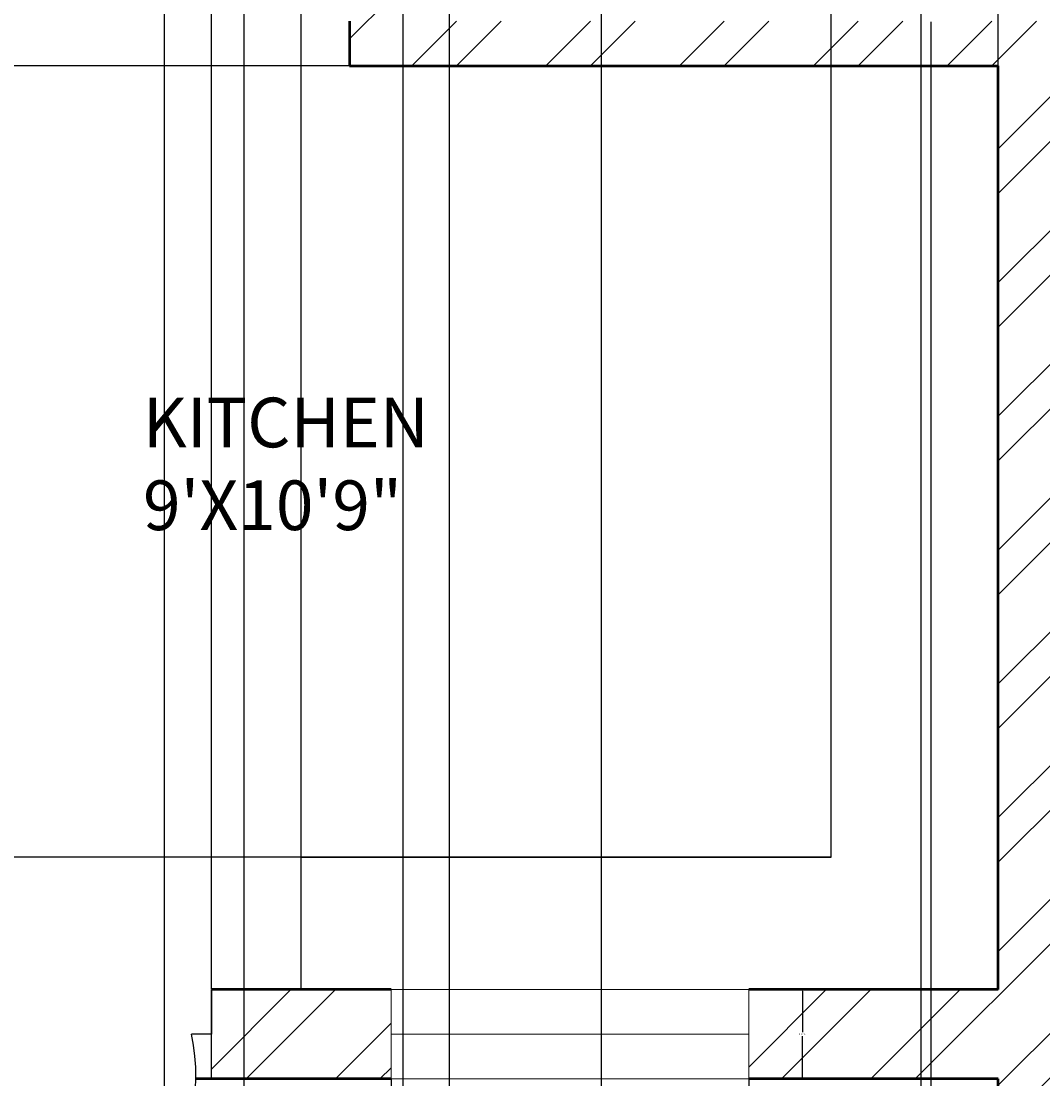
# Model space of a CAD drawing. Units: inches. Extents: x 1980 to 2738, y 1471 to 2568.
# Tile 5 of 22: x 2260 to 2363, y 1686 to 1792. Entities that reach past the tile are written whole.
import ezdxf

# ---------------------------------------------------------------- set-up
doc = ezdxf.new("R2010")
doc.units = ezdxf.units.IN
for name, color, linetype, lineweight in [('A-ANNO-DIMS', 2, 'Continuous', 18), ('A-AREA-IDEN', 7, 'Continuous', 18), ('A-DOOR', 31, 'Continuous', 25), ('A-FLOR-CASE', 8, 'Continuous', 25), ('A-GLAZ', 141, 'Continuous', 18), ('A-WALL', 7, 'Continuous', 50)]:
    doc.layers.add(name, color=color, linetype=linetype, lineweight=lineweight)
doc.layers.add('A-WALL-PATT', color=9, linetype='Continuous', lineweight=13, true_color=0xd19cc7)
doc.styles.get("Standard").update_dxf_attribs({"font": 'arial.ttf'})
doc.dimstyles.get("Standard").update_dxf_attribs({"dimtxt": 0.18, "dimasz": 0.18, "dimexe": 0.18, "dimexo": 0.0625, "dimgap": 0.09, "dimtad": 0, "dimtih": 1, "dimtoh": 1, "dimdec": 4, "dimzin": 0, "dimdsep": 46, "dimtxsty": 'Standard', "dimcen": 0.09, "dimadec": 0, "dimazin": 0, "dimtfac": 1, "dimtdec": 4, "dimtofl": 0, "dimtmove": 0, "dimatfit": 3, "dimfxl": 1, "dimtolj": 1, "dimtzin": 0, "dimarcsym": 0})

# ---------------------------------------------------------------- blocks, each defined once
blk = doc.blocks.new('WIN-36IN-WALL')
for p, q in [((0, 9), (0, 0)), ((0, 9), (36, 9)), ((36, 4.5), (36, 9)), ((36, 9), (36, 0)), ((0, 0), (0, 4.5)), ((0, 4.5), (36, 4.5)), ((36, 0), (0, 0))]:
    blk.add_line(p, q)
blk = doc.blocks.new('*D31')
at = {"layer": 'A-ANNO-DIMS', "color": 0, "lineweight": -2, "transparency": 16777216}
for p, q in [((2297.48, 1685.64), (2297.48, 1680.13)), ((2333.48, 1685.64), (2333.48, 1680.13)), ((2297.66, 1680.31), (2314.36, 1680.31)), ((2333.3, 1680.31), (2316.59, 1680.31))]:
    blk.add_line(p, q, dxfattribs=at)
at = {"layer": 'A-ANNO-DIMS', "color": 0, "transparency": 16777216}
for points in [[(2297.66, 1680.34), (2297.66, 1680.28), (2297.48, 1680.31)], [(2333.3, 1680.34), (2333.3, 1680.28), (2333.48, 1680.31)]]:
    blk.add_solid(points, dxfattribs=at)
at = {"layer": 'Defpoints', "color": 0, "transparency": 16777216}
for p in [(2297.48, 1685.71), (2333.48, 1685.71), (2333.48, 1680.31)]:
    blk.add_point(p, dxfattribs=at)
at = {"layer": 'A-ANNO-DIMS', "color": 0, "transparency": 16777216, "insert": (2315.48, 1680.31), "char_height": 0.18, "attachment_point": 5}
blk.add_mtext('\\A1;WINDOW 36 TYP.', dxfattribs=at)
blk = doc.blocks.new('*D32')
at = {"layer": 'A-ANNO-DIMS', "color": 0, "lineweight": -2, "transparency": 16777216}
for p, q in [((2333.54, 1694.71), (2339.06, 1694.71)), ((2338.88, 1694.53), (2338.88, 1690.39)), ((2338.88, 1685.89), (2338.88, 1690.02)), ((2333.54, 1685.71), (2339.06, 1685.71))]:
    blk.add_line(p, q, dxfattribs=at)
at = {"layer": 'A-ANNO-DIMS', "color": 0, "transparency": 16777216}
for points in [[(2338.85, 1694.53), (2338.91, 1694.53), (2338.88, 1694.71)], [(2338.85, 1685.89), (2338.91, 1685.89), (2338.88, 1685.71)]]:
    blk.add_solid(points, dxfattribs=at)
at = {"layer": 'Defpoints', "color": 0, "transparency": 16777216}
for p in [(2333.48, 1694.71), (2338.88, 1694.71), (2333.48, 1685.71)]:
    blk.add_point(p, dxfattribs=at)
at = {"layer": 'A-ANNO-DIMS', "color": 0, "transparency": 16777216, "insert": (2338.88, 1690.21), "char_height": 0.18, "attachment_point": 5}
blk.add_mtext('\\A1;9 TYP.', dxfattribs=at)
blk = doc.blocks.new('*D40')
at = {"layer": 'A-ANNO-DIMS', "color": 0, "lineweight": -2, "transparency": 16777216}
for p, q in [((2218.65, 2053.14), (2218.65, 1533.71)), ((2298.65, 2053.14), (2298.65, 1533.71)), ((2218.83, 1533.89), (2258.43, 1533.89)), ((2298.47, 1533.89), (2258.87, 1533.89))]:
    blk.add_line(p, q, dxfattribs=at)
at = {"layer": 'A-ANNO-DIMS', "color": 0, "transparency": 16777216}
for points in [[(2218.83, 1533.92), (2218.83, 1533.86), (2218.65, 1533.89)], [(2298.47, 1533.92), (2298.47, 1533.86), (2298.65, 1533.89)]]:
    blk.add_solid(points, dxfattribs=at)
at = {"layer": 'Defpoints', "color": 0, "transparency": 16777216}
for p in [(2218.65, 2053.21), (2298.65, 2053.21), (2298.65, 1533.89)]:
    blk.add_point(p, dxfattribs=at)
at = {"layer": 'A-ANNO-DIMS', "color": 0, "transparency": 16777216, "insert": (2258.65, 1533.89), "char_height": 0.18, "attachment_point": 5}
blk.add_mtext('\\A1;80', dxfattribs=at)
blk = doc.blocks.new('*D41')
at = {"layer": 'A-ANNO-DIMS', "color": 0, "lineweight": -2, "transparency": 16777216}
for p, q in [((2298.65, 2095.14), (2298.65, 1533.71)), ((2515.4, 2095.14), (2515.4, 1533.71)), ((2298.83, 1533.89), (2406.56, 1533.89)), ((2515.22, 1533.89), (2407.49, 1533.89))]:
    blk.add_line(p, q, dxfattribs=at)
at = {"layer": 'A-ANNO-DIMS', "color": 0, "transparency": 16777216}
for points in [[(2298.83, 1533.92), (2298.83, 1533.86), (2298.65, 1533.89)], [(2515.22, 1533.92), (2515.22, 1533.86), (2515.4, 1533.89)]]:
    blk.add_solid(points, dxfattribs=at)
at = {"layer": 'Defpoints', "color": 0, "transparency": 16777216}
for p in [(2298.65, 2095.21), (2515.4, 2095.21), (2515.4, 1533.89)]:
    blk.add_point(p, dxfattribs=at)
at = {"layer": 'A-ANNO-DIMS', "color": 0, "transparency": 16777216, "insert": (2407.03, 1533.89), "char_height": 0.18, "attachment_point": 5}
blk.add_mtext('\\A1;216.75', dxfattribs=at)
blk = doc.blocks.new('*D45')
at = {"layer": 'A-ANNO-DIMS', "color": 0, "lineweight": -2, "transparency": 16777216}
for p, q in [((2255.99, 1694.77), (2255.99, 2507.54)), ((2256.17, 2507.36), (2267.22, 2507.36)), ((2279.21, 2507.36), (2268.15, 2507.36)), ((2279.39, 1694.77), (2279.39, 2507.54))]:
    blk.add_line(p, q, dxfattribs=at)
at = {"layer": 'A-ANNO-DIMS', "color": 0, "transparency": 16777216}
for points in [[(2256.17, 2507.39), (2256.17, 2507.33), (2255.99, 2507.36)], [(2279.21, 2507.39), (2279.21, 2507.33), (2279.39, 2507.36)]]:
    blk.add_solid(points, dxfattribs=at)
at = {"layer": 'Defpoints', "color": 0, "transparency": 16777216}
for p in [(2279.39, 2507.36), (2255.99, 1694.71), (2279.39, 1694.71)]:
    blk.add_point(p, dxfattribs=at)
at = {"layer": 'A-ANNO-DIMS', "color": 0, "transparency": 16777216, "insert": (2267.69, 2507.36), "char_height": 0.18, "attachment_point": 5}
blk.add_mtext('\\A1;23.407', dxfattribs=at)
blk = doc.blocks.new('*D50')
at = {"layer": 'A-ANNO-DIMS', "color": 0, "lineweight": -2, "transparency": 16777216}
for p, q in [((2288.43, 1708.09), (2288.43, 2507.54)), ((2288.61, 2507.36), (2314.71, 2507.36)), ((2341.6, 2507.36), (2315.5, 2507.36)), ((2341.78, 1708.09), (2341.78, 2507.54))]:
    blk.add_line(p, q, dxfattribs=at)
at = {"layer": 'A-ANNO-DIMS', "color": 0, "transparency": 16777216}
for points in [[(2288.61, 2507.39), (2288.61, 2507.33), (2288.43, 2507.36)], [(2341.6, 2507.39), (2341.6, 2507.33), (2341.78, 2507.36)]]:
    blk.add_solid(points, dxfattribs=at)
at = {"layer": 'Defpoints', "color": 0, "transparency": 16777216}
for p in [(2341.78, 2507.36), (2288.43, 1708.03), (2341.78, 1708.03)]:
    blk.add_point(p, dxfattribs=at)
at = {"layer": 'A-ANNO-DIMS', "color": 0, "transparency": 16777216, "insert": (2315.11, 2507.36), "char_height": 0.18, "attachment_point": 5}
blk.add_mtext('\\A1;53.34', dxfattribs=at)
blk = doc.blocks.new('*D51')
at = {"layer": 'A-ANNO-DIMS', "color": 0, "lineweight": -2, "transparency": 16777216}
for p, q in [((2341.78, 1708.09), (2341.78, 2507.54)), ((2341.96, 2507.36), (2349.72, 2507.36)), ((2358.4, 2507.36), (2350.63, 2507.36)), ((2358.58, 1694.77), (2358.58, 2507.54))]:
    blk.add_line(p, q, dxfattribs=at)
at = {"layer": 'A-ANNO-DIMS', "color": 0, "transparency": 16777216}
for points in [[(2341.96, 2507.39), (2341.96, 2507.33), (2341.78, 2507.36)], [(2358.4, 2507.39), (2358.4, 2507.33), (2358.58, 2507.36)]]:
    blk.add_solid(points, dxfattribs=at)
at = {"layer": 'Defpoints', "color": 0, "transparency": 16777216}
for p in [(2358.58, 2507.36), (2341.78, 1708.03), (2358.58, 1694.71)]:
    blk.add_point(p, dxfattribs=at)
at = {"layer": 'A-ANNO-DIMS', "color": 0, "transparency": 16777216, "insert": (2350.18, 2507.36), "char_height": 0.18, "attachment_point": 5}
blk.add_mtext('\\A1;16.807', dxfattribs=at)
blk = doc.blocks.new('*D52')
at = {"layer": 'A-ANNO-DIMS', "color": 0, "lineweight": -2, "transparency": 16777216}
for p, q in [((2341.71, 1787.71), (2036.25, 1787.71)), ((2036.43, 1787.53), (2036.43, 1748.05)), ((2036.43, 1708.21), (2036.43, 1747.69)), ((2341.71, 1708.03), (2036.25, 1708.03))]:
    blk.add_line(p, q, dxfattribs=at)
at = {"layer": 'A-ANNO-DIMS', "color": 0, "transparency": 16777216}
for points in [[(2036.4, 1787.53), (2036.46, 1787.53), (2036.43, 1787.71)], [(2036.4, 1708.21), (2036.46, 1708.21), (2036.43, 1708.03)]]:
    blk.add_solid(points, dxfattribs=at)
at = {"layer": 'Defpoints', "color": 0, "transparency": 16777216}
for p in [(2036.43, 1787.71), (2341.78, 1787.71), (2341.78, 1708.03)]:
    blk.add_point(p, dxfattribs=at)
at = {"layer": 'A-ANNO-DIMS', "color": 0, "transparency": 16777216, "insert": (2036.43, 1747.87), "char_height": 0.18, "attachment_point": 5}
blk.add_mtext('\\A1;79.68', dxfattribs=at)
blk = doc.blocks.new('*D53')
at = {"layer": 'A-ANNO-DIMS', "color": 0, "lineweight": -2, "transparency": 16777216}
for p, q in [((2318.63, 2002.14), (2318.63, 1533.71)), ((2350.79, 2002.14), (2350.79, 1533.71)), ((2318.81, 1533.89), (2334.25, 1533.89)), ((2350.61, 1533.89), (2335.18, 1533.89))]:
    blk.add_line(p, q, dxfattribs=at)
at = {"layer": 'A-ANNO-DIMS', "color": 0, "transparency": 16777216}
for points in [[(2318.81, 1533.92), (2318.81, 1533.86), (2318.63, 1533.89)], [(2350.61, 1533.92), (2350.61, 1533.86), (2350.79, 1533.89)]]:
    blk.add_solid(points, dxfattribs=at)
at = {"layer": 'Defpoints', "color": 0, "transparency": 16777216}
for p in [(2318.63, 2002.21), (2350.79, 2002.21), (2350.79, 1533.89)]:
    blk.add_point(p, dxfattribs=at)
at = {"layer": 'A-ANNO-DIMS', "color": 0, "transparency": 16777216, "insert": (2334.71, 1533.89), "char_height": 0.18, "attachment_point": 5}
blk.add_mtext('\\A1;32.155', dxfattribs=at)
blk = doc.blocks.new('*D57')
at = {"layer": 'A-ANNO-DIMS', "color": 0, "lineweight": -2, "transparency": 16777216}
for p, q in [((2351.81, 1792.14), (2351.81, 1533.71)), ((2372.53, 1792.14), (2372.53, 1533.71)), ((2351.99, 1533.89), (2361.77, 1533.89)), ((2372.35, 1533.89), (2362.56, 1533.89))]:
    blk.add_line(p, q, dxfattribs=at)
at = {"layer": 'A-ANNO-DIMS', "color": 0, "transparency": 16777216}
for points in [[(2351.99, 1533.92), (2351.99, 1533.86), (2351.81, 1533.89)], [(2372.35, 1533.92), (2372.35, 1533.86), (2372.53, 1533.89)]]:
    blk.add_solid(points, dxfattribs=at)
at = {"layer": 'Defpoints', "color": 0, "transparency": 16777216}
for p in [(2351.81, 1792.21), (2372.53, 1792.21), (2372.53, 1533.89)]:
    blk.add_point(p, dxfattribs=at)
at = {"layer": 'A-ANNO-DIMS', "color": 0, "transparency": 16777216, "insert": (2362.17, 1533.89), "char_height": 0.18, "attachment_point": 5}
blk.add_mtext('\\A1;20.72', dxfattribs=at)
blk = doc.blocks.new('*D64')
at = {"layer": 'A-ANNO-DIMS', "color": 0, "lineweight": -2, "transparency": 16777216}
for p, q in [((2303.33, 2002.14), (2303.33, 1533.71)), ((2318.63, 2002.14), (2318.63, 1533.71)), ((2303.51, 1533.89), (2310.67, 1533.89)), ((2318.45, 1533.89), (2311.3, 1533.89))]:
    blk.add_line(p, q, dxfattribs=at)
at = {"layer": 'A-ANNO-DIMS', "color": 0, "transparency": 16777216}
for points in [[(2303.51, 1533.92), (2303.51, 1533.86), (2303.33, 1533.89)], [(2318.45, 1533.92), (2318.45, 1533.86), (2318.63, 1533.89)]]:
    blk.add_solid(points, dxfattribs=at)
at = {"layer": 'Defpoints', "color": 0, "transparency": 16777216}
for p in [(2303.33, 2002.21), (2318.63, 2002.21), (2318.63, 1533.89)]:
    blk.add_point(p, dxfattribs=at)
at = {"layer": 'A-ANNO-DIMS', "color": 0, "transparency": 16777216, "insert": (2310.98, 1533.89), "char_height": 0.18, "attachment_point": 5}
blk.add_mtext('\\A1;15.3', dxfattribs=at)
blk = doc.blocks.new('*D66')
at = {"layer": 'A-ANNO-DIMS', "color": 0, "lineweight": -2, "transparency": 16777216}
for p, q in [((2274.65, 2095.14), (2274.65, 1533.71)), ((2282.65, 2095.14), (2282.65, 1533.71)), ((2274.83, 1533.89), (2278.5, 1533.89)), ((2282.47, 1533.89), (2278.8, 1533.89))]:
    blk.add_line(p, q, dxfattribs=at)
at = {"layer": 'A-ANNO-DIMS', "color": 0, "transparency": 16777216}
for points in [[(2274.83, 1533.92), (2274.83, 1533.86), (2274.65, 1533.89)], [(2282.47, 1533.92), (2282.47, 1533.86), (2282.65, 1533.89)]]:
    blk.add_solid(points, dxfattribs=at)
at = {"layer": 'Defpoints', "color": 0, "transparency": 16777216}
for p in [(2274.65, 2095.21), (2282.65, 2095.21), (2282.65, 1533.89)]:
    blk.add_point(p, dxfattribs=at)
at = {"layer": 'A-ANNO-DIMS', "color": 0, "transparency": 16777216, "insert": (2278.65, 1533.89), "char_height": 0.18, "attachment_point": 5}
blk.add_mtext('\\A1;8', dxfattribs=at)

msp = doc.modelspace()

# ---------------------------------------------------------------- hatches: boundary and pattern name
at = {"layer": 'A-WALL-PATT'}
h = msp.add_hatch(dxfattribs=at)
h.set_pattern_fill('ANSI32', color=256)
h.paths.add_polyline_path([(2257.5661, 2416.2064), (2257.5661, 2420.7064), (2250.5833, 2420.7064), (2250.5833, 2462.7064), (2246.0833, 2462.7064), (2246.0833, 2420.7064), (2237.0791, 2420.7064), (2237.0791, 2411.7064), (2246.0833, 2411.7064), (2246.0833, 2291.7064), (2242.6109, 2291.7064), (2242.6109, 2287.2064), (2246.0833, 2287.2064), (2250.5833, 2287.2064), (2250.5833, 2291.7064), (2250.5833, 2411.7064), (2257.5661, 2411.7064)])
h.paths.add_polyline_path([(2387.0396, 2416.2064), (2387.0396, 2420.7064), (2367.5833, 2420.7064), (2367.5833, 2462.7064), (2358.5833, 2462.7064), (2358.5833, 2420.7064), (2329.3087, 2420.7064), (2329.3087, 2411.7064), (2358.5833, 2411.7064), (2358.5833, 2321.7275), (2358.5833, 2309.7064), (2347.3089, 2309.7064), (2293.3089, 2309.7064), (2293.3089, 2259.0771), (2297.8089, 2259.0771), (2297.8089, 2305.2064), (2347.3089, 2305.2064), (2347.3089, 2284.7412), (2351.8089, 2284.7412), (2351.8089, 2305.2064), (2372.3188, 2305.2064), (2372.3761, 2284.3899), (2377.0295, 2284.3899), (2377.0295, 2299.3058), (2377.0295, 2305.2064), (2426.5295, 2305.2064), (2426.5295, 2257.5573), (2431.0295, 2257.5573), (2431.0295, 2309.7064), (2377.0295, 2309.7064), (2367.5833, 2309.7064), (2367.5833, 2321.7275), (2367.5833, 2411.7064), (2387.0396, 2411.7064)])
h.paths.add_polyline_path([(2448.5267, 2416.2064), (2448.5267, 2420.7064), (2423.0396, 2420.7064), (2423.0396, 2411.7064), (2448.5267, 2411.7064)])
h.paths.add_polyline_path([(2130.9128, 2416.2064), (2130.9128, 2420.7064), (2105.0833, 2420.7064), (2105.0833, 2386.6942), (2114.0833, 2386.6942), (2114.0833, 2411.7064), (2130.9128, 2411.7064)])
h.paths.add_polyline_path([(2212.9478, 2420.7064), (2190.9128, 2420.7064), (2190.9128, 2411.7064), (2212.9478, 2411.7064), (2212.9478, 2416.2064)])
h.paths.add_polyline_path([(2114.0833, 2326.6942), (2105.0833, 2326.6942), (2105.0833, 2291.7064), (2081.0833, 2291.7064), (2081.0833, 2287.2064), (2105.0833, 2287.2064), (2105.0833, 2276.1935), (2114.0833, 2276.1935), (2114.0833, 2287.2064), (2166.3825, 2287.2064), (2166.3825, 2289.4564), (2166.3825, 2291.7064), (2114.0833, 2291.7064)])
h.paths.add_polyline_path([(2114.0833, 2252.1935), (2105.0833, 2252.1935), (2105.0833, 2233.2064), (2081.0833, 2233.2064), (2081.0833, 2228.7064), (2105.0833, 2228.7064), (2105.0833, 2213.4478), (2114.0833, 2213.4478), (2114.0833, 2228.7064), (2195.0833, 2228.7064), (2199.5833, 2228.7064), (2208.4455, 2228.7064), (2208.4455, 2230.9564), (2208.4455, 2233.2064), (2199.5833, 2233.2064), (2199.5833, 2287.2064), (2206.8904, 2287.2064), (2206.8904, 2289.4564), (2206.8904, 2291.7064), (2189.446, 2291.7064), (2189.446, 2289.4564), (2189.446, 2287.2064), (2195.0833, 2287.2064), (2195.0833, 2233.2064), (2114.0833, 2233.2064)])
h.paths.add_polyline_path([(2114.0833, 2153.4478), (2109.5833, 2153.4478), (2105.0833, 2153.4478), (2105.0833, 2135.2374), (2114.0833, 2135.2374)], flags=17)
h.paths.add_polyline_path([(2135.9619, 2095.4081), (2140.1805, 2095.4081), (2140.1805, 2104.2064), (2114.0833, 2104.2064), (2114.0833, 2110.3997), (2109.5833, 2110.3997), (2105.0833, 2110.3997), (2105.0833, 2104.2064), (2081.0833, 2104.2064), (2081.0833, 2099.7064), (2105.0833, 2099.7064), (2127.5416, 2099.8532), (2127.5416, 2056.9393), (2136.2133, 2056.9393)], flags=17)
h.paths.add_polyline_path([(2255.4895, 2104.2064), (2250.5833, 2104.2064), (2250.5833, 2233.2064), (2246.0833, 2233.2064), (2242.4941, 2233.2064), (2242.4941, 2228.7064), (2246.0833, 2228.7064), (2246.0833, 2104.2064), (2163.6825, 2104.2064), (2163.6825, 2099.8072), (2163.6825, 2095.4081), (2191.4325, 2095.4081), (2191.4325, 2011.2064), (2186.0833, 2011.2064), (2136.5143, 2010.8824), (2136.3702, 2032.9403), (2131.9559, 2032.9115), (2127.5416, 2032.8826), (2127.5416, 2006.7064), (2105.0833, 2006.7064), (2081.0833, 2006.7064), (2081.0833, 2002.2064), (2105.0833, 2002.2064), (2105.0833, 1995.9329), (2114.0833, 1995.9329), (2114.0833, 2002.2064), (2246.0833, 2002.2064), (2246.0833, 1877.7064), (2242.1358, 1877.7064), (2242.1358, 1873.2064), (2250.5833, 1873.2064), (2250.5833, 2002.2064), (2255.3335, 2002.2064), (2255.3335, 2011.2064), (2195.9325, 2011.2064), (2195.9325, 2095.2064), (2255.4895, 2095.2064), (2255.4895, 2099.5471)])
h.paths.add_polyline_path([(2199.5833, 1873.2064), (2209.827, 1873.2064), (2209.827, 1875.4564), (2209.827, 1877.7064), (2114.0833, 1877.7064), (2114.0833, 1890.0968), (2105.0833, 1890.0968), (2105.0833, 1877.7064), (2081.0833, 1877.7064), (2081.0833, 1873.2064), (2105.0833, 1873.2064), (2105.0833, 1857.7279), (2114.0833, 1857.7279), (2114.0833, 1873.2064), (2195.0833, 1873.2064), (2195.0833, 1819.2064), (2190.298, 1819.2064), (2190.298, 1814.7064), (2209.8976, 1814.7064), (2209.8976, 1816.9564), (2209.8976, 1819.2064), (2199.5833, 1819.2064)])
h.paths.add_polyline_path([(2114.0833, 1814.7064), (2166.2538, 1814.7064), (2166.2538, 1816.9564), (2166.2538, 1819.2064), (2114.0833, 1819.2064), (2114.0833, 1833.7279), (2109.5833, 1833.7279), (2105.0833, 1833.7279), (2105.0833, 1819.2064), (2081.0833, 1819.2064), (2081.0833, 1814.7064), (2105.0833, 1814.7064), (2105.0833, 1782.5516), (2114.0833, 1782.5516)])
h.paths.add_polyline_path([(2114.0833, 1722.5516), (2109.5833, 1722.5516), (2105.0833, 1722.5516), (2105.0833, 1685.7064), (2124.5104, 1685.7064), (2124.5104, 1690.2064), (2124.5104, 1694.7064), (2114.0833, 1694.7064)])
h.paths.add_polyline_path([(2218.8787, 1694.7064), (2184.5104, 1694.7064), (2184.5104, 1685.7064), (2218.8787, 1685.7064), (2218.8787, 1690.2064)])
h.paths.add_polyline_path([(2250.5833, 1819.2064), (2242.6431, 1819.2064), (2242.6431, 1816.9564), (2242.6431, 1814.7064), (2246.0833, 1814.7064), (2246.0833, 1694.7064), (2240.4035, 1694.7064), (2240.4035, 1690.2064), (2240.4035, 1685.7064), (2246.0833, 1685.7064), (2246.0833, 1643.7064), (2250.5833, 1643.7064), (2250.5833, 1685.7064), (2255.9859, 1685.7064), (2255.9859, 1690.2064), (2255.9859, 1694.7064), (2250.5833, 1694.7064)])
h.paths.add_polyline_path([(2297.4764, 1694.7064), (2279.3934, 1694.7064), (2279.3934, 1690.2064), (2279.3934, 1685.7064), (2297.4764, 1685.7064), (2297.4764, 1690.2064)])
h.paths.add_polyline_path([(2377.1596, 1694.7064), (2367.5833, 1694.7064), (2367.5833, 1787.7064), (2431.0295, 1787.7064), (2431.0295, 1792.2064), (2431.0295, 1849.4149), (2428.7795, 1849.4149), (2426.5295, 1849.4149), (2426.5295, 1792.2064), (2421.5833, 1792.2064), (2367.5833, 1792.2064), (2297.8089, 1792.2064), (2297.8089, 1850.2946), (2295.5589, 1850.2946), (2293.3089, 1850.2946), (2293.3089, 1792.2064), (2293.3089, 1787.7064), (2297.8089, 1787.7064), (2358.5833, 1787.7064), (2358.5833, 1694.7064), (2333.4764, 1694.7064), (2333.4764, 1685.7064), (2358.5833, 1685.7064), (2358.5833, 1643.7064), (2367.5833, 1643.7064), (2367.5833, 1685.7064), (2377.1596, 1685.7064)])
h.paths.add_polyline_path([(2442.4912, 1694.7064), (2413.1596, 1694.7064), (2413.1596, 1685.7064), (2442.4912, 1685.7064)])
h.paths.add_polyline_path([(2480.0833, 1814.7064), (2483.4816, 1814.7064), (2483.4816, 1817.9384), (2483.4816, 1819.2064), (2475.5833, 1819.2064), (2475.5833, 1694.7064), (2470.7283, 1694.7064), (2470.7283, 1685.7064), (2475.5833, 1685.7064), (2475.5833, 1643.7064), (2480.0833, 1643.7064), (2480.0833, 1685.7064), (2486.3293, 1685.7064), (2486.3293, 1690.2064), (2486.3293, 1694.7064), (2480.0833, 1694.7064)])
h.paths.add_polyline_path([(2621.0833, 1721.7349), (2612.0833, 1721.7349), (2612.0833, 1694.7064), (2586.1453, 1694.7064), (2586.1453, 1685.7064), (2621.0833, 1685.7064)])
h.paths.add_polyline_path([(2526.1453, 1690.2064), (2526.1453, 1694.7064), (2511.584, 1694.7064), (2511.584, 1690.2064), (2511.584, 1685.7064), (2526.1453, 1685.7064)])
h.paths.add_polyline_path([(2645.0833, 1819.2064), (2621.0833, 1819.2064), (2621.0833, 1835.8527), (2616.5833, 1835.8527), (2612.0833, 1835.8527), (2612.0833, 1819.2064), (2560.2541, 1819.2064), (2560.2541, 1814.7064), (2612.0833, 1814.7064), (2612.0833, 1781.7349), (2621.0833, 1781.7349), (2621.0833, 1814.7064), (2645.0833, 1814.7064)])
h.paths.add_polyline_path([(2645.0833, 1877.7064), (2621.0833, 1877.7064), (2621.0833, 1886.4375), (2612.0833, 1886.4375), (2612.0833, 1877.7064), (2517.1032, 1877.7064), (2517.1032, 1875.4564), (2517.1032, 1873.2064), (2526.5833, 1873.2064), (2526.5833, 1819.2064), (2516.6454, 1819.2064), (2516.6454, 1816.9564), (2516.6454, 1814.7064), (2536.4445, 1814.7064), (2536.4445, 1816.9564), (2536.4445, 1819.2064), (2531.0833, 1819.2064), (2531.0833, 1873.2064), (2612.0833, 1873.2064), (2612.0833, 1859.8527), (2621.0833, 1859.8527), (2621.0833, 1873.2064), (2645.0833, 1873.2064)])
h.paths.add_polyline_path([(2645.0833, 2006.7064), (2621.0833, 2006.7064), (2588.5085, 2006.7064), (2588.5085, 2052.9125), (2579.9045, 2052.9125), (2579.9045, 2011.2064), (2519.9045, 2011.2064), (2519.9045, 2095.2064), (2553.1204, 2095.2064), (2553.1204, 2104.2064), (2480.0833, 2104.2064), (2480.0833, 2228.7064), (2484.3832, 2228.7064), (2484.3832, 2230.9564), (2484.3832, 2233.2064), (2475.5833, 2233.2064), (2475.5833, 2104.2064), (2463.1308, 2104.2064), (2463.1308, 2095.2064), (2501.2463, 2095.2064), (2510.9045, 2095.2064), (2515.4045, 2095.2064), (2515.4045, 2011.2064), (2510.9045, 2011.2064), (2501.2463, 2011.2064), (2462.5957, 2011.2064), (2462.5957, 2002.2064), (2475.5833, 2002.2064), (2475.5833, 1873.2064), (2483.6146, 1873.2064), (2483.6146, 1875.4564), (2483.6146, 1877.7064), (2480.0833, 1877.7064), (2480.0833, 2002.2064), (2612.0833, 2002.2064), (2612.0833, 1996.309), (2621.0833, 1996.309), (2621.0833, 2002.2064), (2645.0833, 2002.2064)])
h.paths.add_polyline_path([(2588.5085, 2099.7277), (2621.0833, 2099.7277), (2645.0833, 2099.7064), (2645.0833, 2104.2064), (2621.0833, 2104.2064), (2621.0833, 2109.0038), (2616.5833, 2109.0038), (2612.0833, 2109.0038), (2612.0833, 2104.2064), (2575.0621, 2104.2064), (2575.0621, 2099.7064), (2575.0621, 2095.2064), (2579.9045, 2095.2064), (2579.9045, 2076.9125), (2588.5085, 2076.9125)], flags=17)
h.paths.add_polyline_path([(2367.5833, 2002.2064), (2373.7228, 2002.2064), (2373.7228, 2006.7064), (2373.7228, 2011.2064), (2350.7889, 2011.2064), (2350.7889, 2006.7064), (2350.7889, 2002.2064), (2358.5833, 2002.2064), (2358.5833, 1877.7064), (2293.3089, 1877.7064), (2293.3089, 1870.4987), (2297.8089, 1870.4987), (2297.8089, 1873.2064), (2347.3089, 1873.2064), (2347.3089, 1847.2208), (2351.8089, 1847.2208), (2351.8089, 1873.2064), (2372.5295, 1873.2064), (2372.5295, 1847.8619), (2377.0295, 1847.8619), (2377.0295, 1873.2064), (2426.5295, 1873.2064), (2426.5295, 1868.7339), (2431.0295, 1868.7339), (2431.0295, 1877.7064), (2367.5833, 1877.7064)])
h.paths.add_polyline_path([(2531.0833, 2287.2064), (2534.2285, 2287.2064), (2534.2285, 2291.7064), (2516.7886, 2291.7064), (2516.7886, 2287.2064), (2526.5833, 2287.2064), (2526.5833, 2233.2064), (2517.9112, 2233.2064), (2517.9112, 2230.9564), (2517.9112, 2228.7064), (2526.5833, 2228.7064), (2531.0833, 2228.7064), (2612.0833, 2228.7064), (2612.0833, 2206.8504), (2621.0833, 2206.8504), (2621.0833, 2228.7064), (2645.0833, 2228.7064), (2645.0833, 2233.2064), (2621.0833, 2233.2064), (2621.0833, 2241.8536), (2616.5833, 2241.8536), (2612.0833, 2241.8536), (2612.0833, 2233.2064), (2531.0833, 2233.2064)])
h.paths.add_polyline_path([(2645.0833, 2291.7064), (2621.0833, 2291.7064), (2621.0833, 2323.0138), (2616.5833, 2323.0138), (2612.0833, 2323.0138), (2612.0833, 2291.7064), (2559.6852, 2291.7064), (2559.6852, 2289.4564), (2559.6852, 2287.2064), (2612.0833, 2287.2064), (2612.0833, 2265.8536), (2621.0833, 2265.8536), (2621.0833, 2287.2064), (2645.0833, 2287.2064)])
h.paths.add_polyline_path([(2621.0833, 2420.7064), (2582.8189, 2420.7064), (2582.8189, 2411.7064), (2612.0833, 2411.7064), (2612.0833, 2383.0138), (2621.0833, 2383.0138)])
h.paths.add_polyline_path([(2480.0833, 2411.7064), (2485.7342, 2411.7064), (2485.7342, 2416.2064), (2485.7342, 2420.7064), (2480.0833, 2420.7064), (2480.0833, 2462.7064), (2475.5833, 2462.7064), (2475.5833, 2420.7064), (2469.4083, 2420.7064), (2469.4083, 2411.7064), (2475.5833, 2411.7064), (2475.5833, 2291.7064), (2475.5833, 2287.2064), (2482.9195, 2287.2064), (2482.9195, 2289.4564), (2482.9195, 2291.7064), (2480.0833, 2291.7064)])
h.paths.add_polyline_path([(2367.5833, 2228.7064), (2431.0295, 2228.7064), (2431.0295, 2233.2064), (2431.0295, 2237.4203), (2428.7795, 2237.4203), (2426.5295, 2237.4203), (2426.5295, 2233.2064), (2377.0295, 2233.2064), (2377.0295, 2260.3837), (2372.4423, 2260.3837), (2372.517, 2233.2635), (2351.8089, 2233.2064), (2351.8089, 2260.7412), (2347.3089, 2260.7412), (2347.3089, 2233.2064), (2297.8089, 2233.2064), (2297.8089, 2236.9324), (2293.3089, 2236.9324), (2293.3089, 2228.7064), (2358.5833, 2228.7064), (2358.5833, 2104.2064), (2353.3665, 2104.2064), (2353.3665, 2095.2064), (2373.8869, 2095.2064), (2373.8869, 2099.7064), (2373.8869, 2104.2064), (2367.5833, 2104.2064)])
h.paths.add_polyline_path([(2321.2323, 2104.2064), (2303.4895, 2104.2064), (2303.4895, 2095.2064), (2321.2323, 2095.2064), (2321.2323, 2099.7064)], flags=0)
h.paths.add_polyline_path([(2415.1308, 2099.7064), (2415.1308, 2104.2064), (2404.81, 2104.2064), (2404.81, 2095.2064), (2415.1308, 2095.2064)], flags=17)
h.paths.add_polyline_path([(2318.6336, 2011.2064), (2303.3335, 2011.2064), (2303.3335, 2002.2064), (2318.6336, 2002.2064)], flags=0)
h.paths.add_polyline_path([(2414.5957, 2011.2064), (2406.2461, 2011.2064), (2406.2461, 2006.7064), (2406.2461, 2002.2064), (2414.5957, 2002.2064)], flags=17)

# ---------------------------------------------------------------- linework, layer by layer
at = {"layer": 'A-DOOR'}
for p, q in [((2279.3934, 1685.7064), (2279.3934, 1694.7064)), ((2279.3934, 1694.7064), (2279.3934, 1694.7064)), ((2279.3934, 1694.7064), (2279.3934, 1690.2064)), ((2279.3934, 1690.2064), (2277.3934, 1690.2064))]:
    msp.add_line(p, q, dxfattribs=at)
msp.add_arc((2257.9859, 1686.0533), 19.8469, 270, 12.078851, dxfattribs=at)
at = {"layer": 'A-FLOR-CASE'}
for p, q in [((2341.776, 1708.0291), (2341.776, 1787.7064)), ((2288.4349, 1694.7064), (2288.4349, 1708.0291)), ((2288.4349, 1708.0291), (2341.776, 1708.0291))]:
    msp.add_line(p, q, dxfattribs=at)
at = {"layer": 'A-WALL'}
for p, q in [((2293.3089, 1792.2064), (2293.3089, 1787.7064)), ((2293.3089, 1787.7064), (2358.5833, 1787.7064)), ((2293.3089, 1787.7064), (2297.8089, 1787.7064)), ((2358.5833, 1694.7064), (2358.5833, 1787.7064)), ((2297.4764, 1694.7064), (2279.3934, 1694.7064)), ((2358.5833, 1694.7064), (2333.4764, 1694.7064)), ((2297.4764, 1685.7064), (2277.8297, 1685.7064)), ((2358.5833, 1685.7064), (2333.4764, 1685.7064)), ((2358.5833, 1643.7064), (2358.5833, 1685.7064))]:
    msp.add_line(p, q, dxfattribs=at)

# ---------------------------------------------------------------- block references
at = {"layer": 'A-GLAZ'}
msp.add_blockref('WIN-36IN-WALL', (2297.4768, 1685.706), dxfattribs=at)

# ---------------------------------------------------------------- texts
at = {"layer": 'A-AREA-IDEN', "insert": (2272.5068, 1754.2943), "char_height": 5, "width": 77.141965, "attachment_point": 1}
msp.add_mtext('KITCHEN\\P9\'X10\'9"', dxfattribs=at)

# ---------------------------------------------------------------- dimensions: what is measured, and where the dimension line sits
at = {"layer": 'A-ANNO-DIMS'}
for base, p1, p2, override, picture, middle in [((2279.39337, 2507.35642), (2255.98588, 1694.70642), (2279.39337, 1694.70642), {"dimdec": 3, "dimlfac": 1, "dimrnd": 0, "dimzin": 0, "dimdsep": 46, "dimlunit": 2}, '*D45', (2267.68962, 2507.35642)), ((2341.776, 2507.3564), (2288.4349, 1708.0291), (2341.776, 1708.0291), {"dimdec": 2, "dimlfac": 1, "dimrnd": 0, "dimzin": 0, "dimdsep": 46, "dimlunit": 2}, '*D50', (2315.1054, 2507.3564)), ((2358.5833, 2507.3564), (2341.776, 1708.0291), (2358.5833, 1694.7064), {"dimdec": 3, "dimlfac": 1, "dimrnd": 0, "dimzin": 0, "dimdsep": 46, "dimlunit": 2}, '*D51', (2350.1796, 2507.3564)), ((2282.6516, 1533.8857), (2274.6516, 2095.2064), (2282.6516, 2095.2064), {"dimdec": 0, "dimlfac": 1, "dimrnd": 0, "dimzin": 0, "dimdsep": 46, "dimlunit": 2}, '*D66', (2278.6516, 1533.8857)), ((2515.4045, 1533.8857), (2298.6516, 2095.2064), (2515.4045, 2095.2064), {"dimdec": 2, "dimlfac": 1, "dimrnd": 0, "dimzin": 0, "dimdsep": 46, "dimlunit": 2}, '*D41', (2407.0281, 1533.8857)), ((2298.6516, 1533.8857), (2218.6516, 2053.2064), (2298.6516, 2053.2064), {"dimdec": 0, "dimlfac": 1, "dimrnd": 0, "dimzin": 0, "dimdsep": 46, "dimlunit": 2}, '*D40', (2258.6516, 1533.8857)), ((2318.6336, 1533.8857), (2303.3335, 2002.2064), (2318.6336, 2002.2064), {"dimdec": 1, "dimlfac": 1, "dimrnd": 0, "dimzin": 0, "dimdsep": 46, "dimlunit": 2}, '*D64', (2310.9835, 1533.8857)), ((2350.7889, 1533.8857), (2318.6336, 2002.2064), (2350.7889, 2002.2064), {"dimdec": 3, "dimlfac": 1, "dimrnd": 0, "dimzin": 0, "dimdsep": 46, "dimlunit": 2}, '*D53', (2334.7112, 1533.8857)), ((2372.5295, 1533.8857), (2351.8089, 1792.2064), (2372.5295, 1792.2064), {"dimdec": 2, "dimlfac": 1, "dimrnd": 0, "dimzin": 0, "dimdsep": 46, "dimlunit": 2}, '*D57', (2362.1692, 1533.8857))]:
    dim = msp.add_linear_dim(base=base, p1=p1, p2=p2, dimstyle='Standard', override=override, dxfattribs=at)
    dim.commit()
    dim.dimension.update_dxf_attribs({"geometry": picture, "text_midpoint": middle})
dim = msp.add_linear_dim(base=(2036.4333, 1787.7064), p1=(2341.776, 1708.0291), p2=(2341.776, 1787.7064), angle=90, dimstyle='Standard', override={"dimdec": 2, "dimlfac": 1, "dimrnd": 0, "dimzin": 0, "dimdsep": 46, "dimlunit": 2}, dxfattribs=at)
dim.commit()
dim.dimension.update_dxf_attribs({"geometry": '*D52', "text_midpoint": (2036.4333, 1747.8678)})
dim = msp.add_linear_dim(base=(2338.8764, 1694.7064), p1=(2333.4764, 1685.7064), p2=(2333.4764, 1694.7064), angle=90, text='<> TYP.', dimstyle='Standard', override={"dimdec": 0, "dimlfac": 1, "dimrnd": 0, "dimzin": 0, "dimdsep": 46, "dimlunit": 2}, dxfattribs=at)
dim.commit()
dim.dimension.update_dxf_attribs({"geometry": '*D32', "text_midpoint": (2338.8764, 1690.2064)})
dim = msp.add_linear_dim(base=(2333.4764, 1680.3064), p1=(2297.4764, 1685.7064), p2=(2333.4764, 1685.7064), text='WINDOW <> TYP.', dimstyle='Standard', override={"dimdec": 0, "dimlfac": 1, "dimrnd": 0, "dimzin": 0, "dimdsep": 46, "dimlunit": 2}, dxfattribs=at)
dim.commit()
dim.dimension.update_dxf_attribs({"geometry": '*D31', "text_midpoint": (2315.4764, 1680.3064)})

doc.saveas('drawing.dxf')
